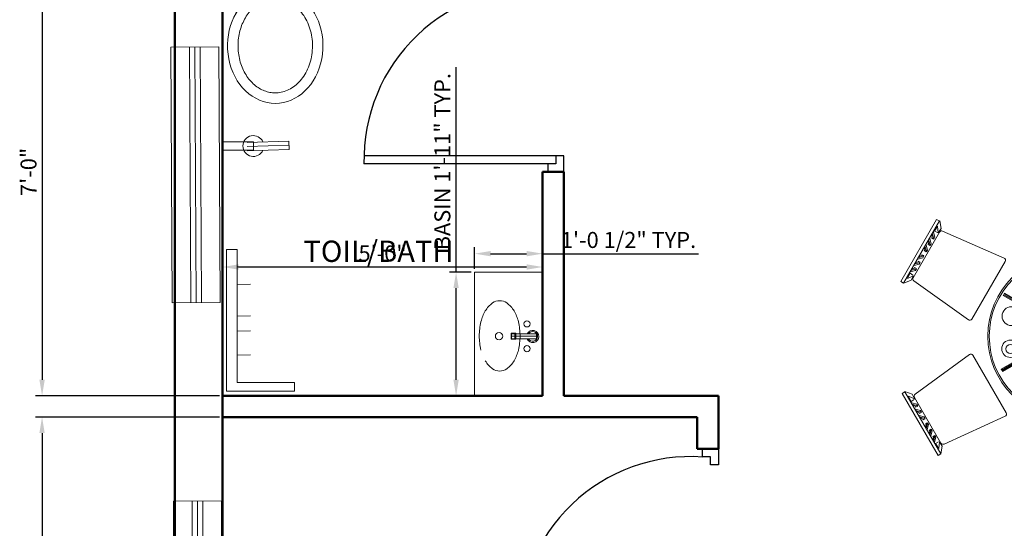
# Model space of a CAD drawing. Units: inches. Extents: x 108 to 1546, y -229 to 513.
# Tile 9 of 11: x 1167 to 1352, y 187 to 282. Entities that reach past the tile are written whole.
import ezdxf

# ---------------------------------------------------------------- set-up
doc = ezdxf.new("R2010")
doc.units = ezdxf.units.IN
for name, color, linetype, lineweight in [('A-ANNO-DIMS', 2, 'Continuous', 18), ('A-AREA-IDEN', 4, 'Continuous', 18), ('A-FLOR-FIXT', 9, 'Continuous', 18), ('A-FURN', 8, 'Continuous', 13), ('door', 1, 'Continuous', 25), ('wall', 7, 'Continuous', 50), ('WINDOW', 212, 'Continuous', 18)]:
    doc.layers.add(name, color=color, linetype=linetype, lineweight=lineweight)
doc.styles.get("Standard").update_dxf_attribs({"font": 'arial.ttf'})
doc.dimstyles.new('ISO-25', dxfattribs={"dimtxt": 3, "dimasz": 3, "dimexe": 1.25, "dimexo": 0.625, "dimtad": 1, "dimdec": 1, "dimlunit": 3, "dimtxsty": 'Standard', "dimcen": 2.5, "dimadec": 0, "dimazin": 0, "dimtfac": 1, "dimtdec": 1, "dimtmove": 0, "dimatfit": 3, "dimfxl": 1, "dimarcsym": 0})

# ---------------------------------------------------------------- blocks, each defined once
blk = doc.blocks.new('A$C45501D90')
for p, q in [((-242.2, 1133.5), (224, 1133.5)), ((-242.2, 1112.8), (-242.2, 1133.5)), ((224, 1112.8), (-242.2, 1112.8)), ((-242.2, 1111.2), (-202.3, 1079.2)), ((-203.9, 1106.4), (-165.6, 1108)), ((-168.8, 1080.8), (-203.9, 1106.4)), ((-165.6, 1108), (-167.2, 1085.6)), ((-156, 1109.6), (-132, 1085.6)), ((-119.3, 1085.6), (-143.2, 1108)), ((-143.2, 1108), (-133.6, 1108)), ((-133.6, 1108), (-122.5, 1098.4)), ((-122.5, 1098.4), (-119.3, 1101.6)), ((-119.3, 1101.6), (-117.7, 1087.2)), ((-108.1, 1109.6), (-84.1, 1085.6)), ((-71.4, 1085.6), (-95.3, 1108)), ((-95.3, 1108), (-85.7, 1108)), ((-85.7, 1108), (-74.6, 1098.4)), ((-74.6, 1098.4), (-71.4, 1101.6)), ((-71.4, 1101.6), (-69.8, 1087.2)), ((-60.2, 1109.6), (-36.2, 1085.6)), ((-23.5, 1085.6), (-47.4, 1108)), ((-47.4, 1108), (-37.8, 1108)), ((-37.8, 1108), (-26.7, 1098.4)), ((-26.7, 1098.4), (-23.5, 1101.6)), ((-23.5, 1101.6), (-21.9, 1087.2)), ((8.5, 1101.6), (6.9, 1087.2)), ((8.5, 1085.6), (32.4, 1108)), ((11.6, 1098.4), (8.5, 1101.6)), ((22.8, 1108), (11.6, 1098.4)), ((45.2, 1109.6), (21.2, 1085.6)), ((32.4, 1108), (22.8, 1108)), ((56.3, 1101.6), (54.8, 1087.2)), ((56.3, 1085.6), (80.3, 1108)), ((59.5, 1098.4), (56.3, 1101.6)), ((70.7, 1108), (59.5, 1098.4)), ((93.1, 1109.6), (69.1, 1085.6)), ((80.3, 1108), (70.7, 1108)), ((104.2, 1101.6), (102.6, 1087.2)), ((104.2, 1085.6), (128.2, 1108)), ((107.4, 1098.4), (104.2, 1101.6)), ((118.6, 1108), (107.4, 1098.4)), ((141, 1109.6), (117, 1085.6)), ((128.2, 1108), (118.6, 1108)), ((188.9, 1106.4), (150.5, 1108)), ((150.5, 1108), (152.1, 1085.6)), ((153.7, 1080.8), (188.9, 1106.4)), ((224, 1112.8), (187.3, 1079.2)), ((224, 1133.5), (224, 1112.8)), ((-197.3, 1061.6), (-238.9, 627.6)), ((-202.3, 1079.2), (-168.8, 1080.8)), ((161.8, 1076.1), (-181.4, 1076.1)), ((-132, 1085.6), (-119.3, 1085.6)), ((-84.1, 1085.6), (-71.4, 1085.6)), ((-36.2, 1085.6), (-23.5, 1085.6)), ((21.2, 1085.6), (8.5, 1085.6)), ((69.1, 1085.6), (56.3, 1085.6)), ((117, 1085.6), (104.2, 1085.6)), ((187.3, 1079.2), (153.7, 1080.8)), ((225.2, 627.8), (177.6, 1061.8)), ((842.6, 766.1), (860.5, 776.5)), ((860.5, 776.5), (1093.6, 372.8)), ((-1102.7, 357), (-869.7, 760.7)), ((-851.7, 750.4), (-1084.8, 346.6)), ((-863.7, 716.7), (-884.3, 684.4)), ((-869.7, 760.7), (-851.7, 750.4)), ((-859.2, 673.6), (-863.7, 716.7)), ((-848.7, 752.3), (-841, 701.8)), ((841.2, 765.3), (833.5, 714.8)), ((833.5, 714.8), (851.7, 686.6)), ((1075.7, 362.4), (842.6, 766.1)), ((851.7, 686.6), (856.2, 729.8)), ((856.2, 729.8), (876.7, 697.4)), ((-851, 678.1), (-1022.6, 380.9)), ((-897.5, 642.2), (-901.9, 641.1)), ((-901.9, 641.1), (-890.2, 632.5)), ((-895.4, 665), (-900.2, 656.7)), ((-900.2, 656.7), (-897.5, 642.2)), ((-888.1, 633.1), (-895.4, 665)), ((-890.4, 676.9), (-881.7, 644.2)), ((-881.7, 644.2), (-888.1, 633.1)), ((-884.3, 684.4), (-864.1, 674.6)), ((-841, 701.8), (-859.2, 673.6)), ((-431.1, 509), (-830.8, 684.8)), ((820.7, 701.7), (424.1, 520.7)), ((1012.8, 397.9), (841.2, 695.1)), ((876.7, 697.4), (856.6, 687.6)), ((882.9, 689.9), (874.2, 657.2)), ((874.2, 657.2), (880.6, 646.1)), ((880.6, 646.1), (887.9, 678)), ((894.4, 654.1), (882.7, 645.5)), ((887.9, 678), (892.7, 669.7)), ((892.7, 669.7), (890, 655.2)), ((890, 655.2), (894.4, 654.1)), ((906.9, 648.4), (898.1, 615.7)), ((-943.3, 582), (-948.1, 573.8)), ((-936, 550.1), (-943.3, 582)), ((-938.3, 593.9), (-929.6, 561.2)), ((-921.5, 600.8), (-925.8, 599.6)), ((-925.8, 599.6), (-914.2, 591)), ((-919.4, 623.5), (-924.2, 615.2)), ((-924.2, 615.2), (-921.5, 600.8)), ((-912, 591.6), (-919.4, 623.5)), ((-914.4, 635.4), (-905.6, 602.7)), ((-905.6, 602.7), (-912, 591.6)), ((-223, 610.1), (209.4, 610.1)), ((898.1, 615.7), (904.5, 604.6)), ((904.5, 604.6), (911.9, 636.5)), ((918.3, 612.6), (906.7, 604)), ((911.9, 636.5), (916.7, 628.2)), ((916.7, 628.2), (914, 613.8)), ((914, 613.8), (918.3, 612.6)), ((930.8, 606.9), (922.1, 574.2)), ((928.4, 563.1), (935.8, 595.1)), ((935.8, 595.1), (940.6, 586.8)), ((940.6, 586.8), (937.9, 572.3)), ((-951.9, 522.5), (-983.2, 512.9)), ((-983.2, 512.9), (-978.5, 521.2)), ((-978.5, 521.2), (-964.6, 526.1)), ((-964.6, 526.1), (-965.7, 530.5)), ((-965.7, 530.5), (-952.5, 524.7)), ((-958.3, 511.4), (-951.9, 522.5)), ((-945.4, 559.3), (-949.8, 558.1)), ((-949.8, 558.1), (-938.1, 549.6)), ((-948.1, 573.8), (-945.4, 559.3)), ((-929.6, 561.2), (-936, 550.1)), ((922.1, 574.2), (928.4, 563.1)), ((942.3, 571.1), (930.6, 562.6)), ((937.9, 572.3), (942.3, 571.1)), ((950.8, 524.4), (944.4, 535.5)), ((944.4, 535.5), (975.7, 525.9)), ((958.2, 543.5), (945, 537.7)), ((983.5, 515.7), (950.8, 524.4)), ((957.1, 539.1), (958.2, 543.5)), ((970.9, 534.2), (957.1, 539.1)), ((975.7, 525.9), (970.9, 534.2)), ((-1015, 461.2), (-982.3, 469.9)), ((-975.9, 481), (-1007.2, 471.4)), ((-1007.2, 471.4), (-1002.4, 479.7)), ((-1002.4, 479.7), (-988.5, 484.6)), ((-991, 502.7), (-958.3, 511.4)), ((-988.5, 484.6), (-989.7, 489)), ((-989.7, 489), (-976.5, 483.2)), ((-982.3, 469.9), (-975.9, 481)), ((-639.9, 111.9), (-423.7, 486.4)), ((-5.6, 508.7, 90.8), (0.4, 508.7, 90.8)), ((-5.6, 317.7, 90.8), (-5.6, 508.7, 90.8)), ((0.4, 508.7, 90.8), (0.4, 317.7, 90.8)), ((5.8, 317.7, 90.8), (5.8, 508.7, 90.8)), ((5.8, 508.7, 90.8), (11.8, 508.7, 90.8)), ((11.8, 508.7, 90.8), (11.8, 317.7, 90.8)), ((416.9, 498.2), (633.1, 123.7)), ((968.4, 494), (999.7, 484.4)), ((974.7, 483), (968.4, 494)), ((982.2, 502), (968.9, 496.2)), ((1007.4, 474.2), (974.7, 483)), ((981, 497.6), (982.2, 502)), ((994.9, 492.7), (981, 497.6)), ((998.7, 441.5), (992.3, 452.5)), ((992.3, 452.5), (1023.6, 443)), ((1006.1, 460.5), (992.9, 454.7)), ((999.7, 484.4), (994.9, 492.7)), ((1005, 456.2), (1006.1, 460.5)), ((1018.8, 451.3), (1005, 456.2)), ((1023.6, 443), (1018.8, 451.3)), ((-1060.1, 376.6), (-1042.3, 410.6)), ((-1020.4, 394.3), (-1060.1, 376.6)), ((-1042.3, 410.6), (-1023.8, 398.1)), ((-1038.9, 419.7), (-1006.2, 428.5)), ((-1035.8, 364.4), (-1020.4, 394.3)), ((-999.8, 439.5), (-1031.1, 430)), ((-1031.1, 430), (-1026.3, 438.3)), ((-1026.3, 438.3), (-1012.5, 443.1)), ((-1012.5, 443.1), (-1013.6, 447.5)), ((-1013.6, 447.5), (-1000.4, 441.7)), ((-1006.2, 428.5), (-999.8, 439.5)), ((1031.4, 432.7), (998.7, 441.5)), ((1028.3, 377.5), (1012.9, 407.3)), ((1012.9, 407.3), (1052.6, 389.6)), ((1034.8, 423.6), (1016.3, 411.1)), ((1052.6, 389.6), (1034.8, 423.6)), ((-1084.8, 346.6), (-1102.7, 357)), ((-1083.4, 345.8), (-1035.8, 364.4)), ((-1018, 360), (-663, 106.9)), ((-22.3, 329.1, 90.8), (-22.3, 344.6, 90.8)), ((-22.3, 344.6, 90.8), (-5.6, 344.6, 90.8)), ((-5.6, 329.1, 90.8), (-22.3, 329.1, 90.8)), ((0.4, 344.6, 90.8), (5.8, 344.6, 90.8)), ((5.8, 329.1, 90.8), (0.4, 329.1, 90.8)), ((11.8, 344.6, 90.8), (27.3, 344.6, 90.8)), ((27.3, 329.1, 90.8), (11.8, 329.1, 90.8)), ((27.3, 344.6, 90.8), (27.3, 329.1, 90.8)), ((656.3, 118.9), (1008.4, 377.1)), ((1075.9, 358.8), (1028.3, 377.5)), ((1093.6, 372.8), (1075.7, 362.4)), ((-436.3, 265.3, 90.8), (-433.3, 270.5, 90.8)), ((-270.9, 169.9, 90.8), (-436.3, 265.3, 90.8)), ((-433.3, 270.5, 90.8), (-267.9, 175, 90.8)), ((-430.6, 275.2, 90.8), (-427.6, 280.3, 90.8)), ((-265.2, 179.7, 90.8), (-430.6, 275.2, 90.8)), ((-427.6, 280.3, 90.8), (-262.3, 184.9, 90.8)), ((-175.3, 276.1, 90.8), (-104.8, 293.2, 90.8)), ((-103.3, 252.4, 90.8), (-175.3, 276.1, 90.8)), ((-104.8, 293.2, 90.8), (-85.5, 278.4, 90.8)), ((-85.5, 278.4, 90.8), (-52.1, 293.9, 90.8)), ((9.5, 276.1, 90.8), (-59.5, 246.5, 90.8)), ((-52.1, 293.9, 90.8), (9.5, 276.1, 90.8)), ((0.4, 317.7, 90.8), (-5.6, 317.7, 90.8)), ((11.8, 317.7, 90.8), (5.8, 317.7, 90.8)), ((134.3, 288, 90.8), (184.3, 235.5, 90.8)), ((149.7, 213.9, 90.8), (134.3, 288, 90.8)), ((255.2, 161.9, 90.8), (420.6, 257.3, 90.8)), ((420.6, 257.3, 90.8), (423.5, 252.2, 90.8)), ((-291.2, 188.5, 90.8), (-288.5, 193.1, 90.8)), ((-285.5, 198.3, 90.8), (-277.8, 211.7, 90.8)), ((-277.8, 211.7, 90.8), (-264.3, 204, 90.8)), ((-264.3, 204, 90.8), (-272.1, 190.5, 90.8)), ((-59.5, 246.5, 90.8), (-103.3, 252.4, 90.8)), ((166.5, 173, 90.8), (149.7, 213.9, 90.8)), ((184.3, 235.5, 90.8), (181.1, 211.4, 90.8)), ((181.1, 211.4, 90.8), (211.3, 190.3, 90.8)), ((423.5, 252.2, 90.8), (258.2, 156.7, 90.8)), ((260.9, 152, 90.8), (426.2, 247.5, 90.8)), ((429.2, 242.3, 90.8), (263.8, 146.9, 90.8)), ((426.2, 247.5, 90.8), (429.2, 242.3, 90.8)), ((-302.5, 168.8, 90.8), (-294.2, 183.3, 90.8)), ((-289.1, 161.1, 90.8), (-302.5, 168.8, 90.8)), ((-280.7, 175.5, 90.8), (-289.1, 161.1, 90.8)), ((-275.1, 185.4, 90.8), (-277.8, 180.7, 90.8)), ((-273.6, 117.6, 90.8), (-227.4, 162.1, 90.8)), ((-267.9, 175, 90.8), (-270.9, 169.9, 90.8)), ((-262.3, 184.9, 90.8), (-265.2, 179.7, 90.8)), ((-227.4, 162.1, 90.8), (-236.2, 87.5, 90.8)), ((226.7, 128.1, 90.8), (166.5, 173, 90.8)), ((211.3, 190.3, 90.8), (226.7, 128.1, 90.8)), ((258.2, 156.7, 90.8), (255.2, 161.9, 90.8)), ((256.6, 182, 90.8), (270.1, 189.8, 90.8)), ((265, 167.5, 90.8), (256.6, 182, 90.8)), ((263.8, 146.9, 90.8), (260.9, 152, 90.8)), ((270.7, 157.7, 90.8), (268, 162.4, 90.8)), ((270.1, 189.8, 90.8), (278.4, 175.3, 90.8)), ((281.4, 139.1, 90.8), (273.7, 152.5, 90.8)), ((281.4, 170.1, 90.8), (284.1, 165.5, 90.8)), ((294.9, 146.8, 90.8), (281.4, 139.1, 90.8)), ((287.1, 160.3, 90.8), (294.9, 146.8, 90.8)), ((-319.8, 2.1, 90.8), (-299.3, 71.7, 90.8)), ((-299.3, 71.7, 90.8), (-276.8, 80.9, 90.8)), ((-276.8, 80.9, 90.8), (-273.6, 117.6, 90.8)), ((-236.2, 87.5, 90.8), (-263.2, 52.5, 90.8)), ((-263.2, 52.5, 90.8), (-319.8, 2.1, 90.8)), ((242.9, -24.6, 90.8), (299.4, 25.9, 90.8)), ((299.4, 25.9, 90.8), (278.9, -43.7, 90.8)), ((207, -134.1, 90.8), (215.8, -59.5, 90.8)), ((215.8, -59.5, 90.8), (242.9, -24.6, 90.8)), ((256.4, -53, 90.8), (253.2, -89.7, 90.8)), ((278.9, -43.7, 90.8), (256.4, -53, 90.8)), ((-656.3, -118.9), (-1008.4, -377.1)), ((-416.9, -498.2), (-633.1, -123.7)), ((-449.6, -214.4, 90.8), (-284.2, -118.9, 90.8)), ((-281.2, -124.1, 90.8), (-446.6, -219.5, 90.8)), ((-315.2, -118.9, 90.8), (-301.8, -111.1, 90.8)), ((-307.5, -132.3, 90.8), (-315.2, -118.9, 90.8)), ((-301.8, -111.1, 90.8), (-294, -124.6, 90.8)), ((-284.2, -118.9, 90.8), (-281.2, -124.1, 90.8)), ((-247, -100.1, 90.8), (-186.8, -145, 90.8)), ((-231.7, -162.3, 90.8), (-247, -100.1, 90.8)), ((253.2, -89.7, 90.8), (207, -134.1, 90.8)), ((639.9, -111.9), (423.7, -486.4)), ((1018, -360), (663, -106.9)), ((-443.9, -224.2, 90.8), (-278.5, -128.7, 90.8)), ((-275.5, -133.9, 90.8), (-440.9, -229.4, 90.8)), ((-301.8, -142.1, 90.8), (-304.5, -137.5, 90.8)), ((-290.4, -161.8, 90.8), (-298.8, -147.3, 90.8)), ((-291, -129.7, 90.8), (-288.3, -134.4, 90.8)), ((-277, -154, 90.8), (-290.4, -161.8, 90.8)), ((-285.4, -139.5, 90.8), (-277, -154, 90.8)), ((-278.5, -128.7, 90.8), (-275.5, -133.9, 90.8)), ((-201.5, -183.4, 90.8), (-231.7, -162.3, 90.8)), ((-204.7, -207.6, 90.8), (-201.5, -183.4, 90.8)), ((-186.8, -145, 90.8), (-170.1, -185.9, 90.8)), ((-170.1, -185.9, 90.8), (-154.7, -260.1, 90.8)), ((241.9, -156.9, 90.8), (244.9, -151.7, 90.8)), ((407.3, -252.4, 90.8), (241.9, -156.9, 90.8)), ((244, -176, 90.8), (251.7, -162.5, 90.8)), ((257.4, -183.7, 90.8), (244, -176, 90.8)), ((244.9, -151.7, 90.8), (410.3, -247.2, 90.8)), ((247.6, -147.1, 90.8), (250.6, -141.9, 90.8)), ((413, -242.5, 90.8), (247.6, -147.1, 90.8)), ((250.6, -141.9, 90.8), (415.9, -237.4, 90.8)), ((254.7, -157.4, 90.8), (257.4, -152.7, 90.8)), ((265.2, -170.3, 90.8), (257.4, -183.7, 90.8)), ((260.4, -147.6, 90.8), (268.7, -133.1, 90.8)), ((270.8, -160.5, 90.8), (268.1, -165.1, 90.8)), ((268.7, -133.1, 90.8), (282.2, -140.8, 90.8)), ((282.2, -140.8, 90.8), (273.8, -155.3, 90.8)), ((-446.6, -219.5, 90.8), (-449.6, -214.4, 90.8)), ((-440.9, -229.4, 90.8), (-443.9, -224.2, 90.8)), ((-154.7, -260.1, 90.8), (-204.7, -207.6, 90.8)), ((-29.8, -248.2, 90.8), (39.2, -218.5, 90.8)), ((31.8, -266, 90.8), (-29.8, -248.2, 90.8)), ((65.2, -250.4, 90.8), (31.8, -266, 90.8)), ((39.2, -218.5, 90.8), (83, -224.4, 90.8)), ((84.4, -265.2, 90.8), (65.2, -250.4, 90.8)), ((83, -224.4, 90.8), (154.9, -248.2, 90.8)), ((154.9, -248.2, 90.8), (84.4, -265.2, 90.8)), ((410.3, -247.2, 90.8), (407.3, -252.4, 90.8)), ((415.9, -237.4, 90.8), (413, -242.5, 90.8)), ((-47.6, -316.6, 90.8), (-47.6, -301.1, 90.8)), ((-47.6, -301.1, 90.8), (-32.1, -301.1, 90.8)), ((-32.1, -316.6, 90.8), (-47.6, -316.6, 90.8)), ((-32.1, -480.7, 90.8), (-32.1, -289.8, 90.8)), ((-32.1, -289.8, 90.8), (-26.1, -289.8, 90.8)), ((-26.1, -289.8, 90.8), (-26.1, -480.7, 90.8)), ((-26.1, -301.1, 90.8), (-20.8, -301.1, 90.8)), ((-20.8, -316.6, 90.8), (-26.1, -316.6, 90.8)), ((-20.8, -480.7, 90.8), (-20.8, -289.8, 90.8)), ((-20.8, -289.8, 90.8), (-14.8, -289.8, 90.8)), ((-14.8, -289.8, 90.8), (-14.8, -480.7, 90.8)), ((-14.8, -301.1, 90.8), (1.9, -301.1, 90.8)), ((1.9, -316.6, 90.8), (-14.8, -316.6, 90.8)), ((1.9, -301.1, 90.8), (1.9, -316.6, 90.8)), ((-1093.6, -372.8), (-1075.7, -362.4)), ((-860.5, -776.5), (-1093.6, -372.8)), ((-1075.9, -358.8), (-1028.3, -377.5)), ((-1075.7, -362.4), (-842.6, -766.1)), ((-1028.3, -377.5), (-1012.9, -407.3)), ((851, -678.1), (1022.6, -380.9)), ((851.7, -750.4), (1084.8, -346.6)), ((1102.7, -357), (869.7, -760.7)), ((1035.8, -364.4), (1020.4, -394.3)), ((1020.4, -394.3), (1060.1, -376.6)), ((1083.4, -345.8), (1035.8, -364.4)), ((1060.1, -376.6), (1042.3, -410.6)), ((1084.8, -346.6), (1102.7, -357)), ((-1052.6, -389.6), (-1034.8, -423.6)), ((-1012.9, -407.3), (-1052.6, -389.6)), ((-1034.8, -423.6), (-1016.3, -411.1)), ((-1031.4, -432.7), (-998.7, -441.5)), ((-1023.6, -443), (-1018.8, -451.3)), ((-992.3, -452.5), (-1023.6, -443)), ((-1012.8, -397.9), (-841.2, -695.1)), ((-998.7, -441.5), (-992.3, -452.5)), ((1006.2, -428.5), (999.8, -439.5)), ((999.8, -439.5), (1031.1, -430)), ((1013.6, -447.5), (1000.4, -441.7)), ((1038.9, -419.7), (1006.2, -428.5)), ((1026.3, -438.3), (1012.5, -443.1)), ((1012.5, -443.1), (1013.6, -447.5)), ((1042.3, -410.6), (1023.8, -398.1)), ((1031.1, -430), (1026.3, -438.3)), ((-1018.8, -451.3), (-1005, -456.2)), ((-1007.4, -474.2), (-974.7, -483)), ((-1006.1, -460.5), (-992.9, -454.7)), ((-1005, -456.2), (-1006.1, -460.5)), ((-968.4, -494), (-999.7, -484.4)), ((-999.7, -484.4), (-994.9, -492.7)), ((-994.9, -492.7), (-981, -497.6)), ((-982.2, -502), (-968.9, -496.2)), ((-981, -497.6), (-982.2, -502)), ((-974.7, -483), (-968.4, -494)), ((-26.1, -480.7, 90.8), (-32.1, -480.7, 90.8)), ((-14.8, -480.7, 90.8), (-20.8, -480.7, 90.8)), ((431.1, -509), (830.8, -684.8)), ((958.3, -511.4), (951.9, -522.5)), ((991, -502.7), (958.3, -511.4)), ((982.3, -469.9), (975.9, -481)), ((975.9, -481), (1007.2, -471.4)), ((989.7, -489), (976.5, -483.2)), ((1015, -461.2), (982.3, -469.9)), ((1002.4, -479.7), (988.5, -484.6)), ((988.5, -484.6), (989.7, -489)), ((1007.2, -471.4), (1002.4, -479.7)), ((-983.5, -515.7), (-950.8, -524.4)), ((-944.4, -535.5), (-975.7, -525.9)), ((-975.7, -525.9), (-970.9, -534.2)), ((-970.9, -534.2), (-957.1, -539.1)), ((-958.2, -543.5), (-945, -537.7)), ((-957.1, -539.1), (-958.2, -543.5)), ((-950.8, -524.4), (-944.4, -535.5)), ((-942.3, -571.1), (-930.6, -562.6)), ((-937.9, -572.3), (-942.3, -571.1)), ((-940.6, -586.8), (-937.9, -572.3)), ((-928.4, -563.1), (-935.8, -595.1)), ((-930.8, -606.9), (-922.1, -574.2)), ((-922.1, -574.2), (-928.4, -563.1)), ((-820.7, -701.7), (-424.1, -520.7)), ((929.6, -561.2), (936, -550.1)), ((938.3, -593.9), (929.6, -561.2)), ((936, -550.1), (943.3, -582)), ((949.8, -558.1), (938.1, -549.6)), ((943.3, -582), (948.1, -573.8)), ((945.4, -559.3), (949.8, -558.1)), ((948.1, -573.8), (945.4, -559.3)), ((951.9, -522.5), (983.2, -512.9)), ((965.7, -530.5), (952.5, -524.7)), ((978.5, -521.2), (964.6, -526.1)), ((964.6, -526.1), (965.7, -530.5)), ((983.2, -512.9), (978.5, -521.2)), ((-935.8, -595.1), (-940.6, -586.8)), ((-918.3, -612.6), (-906.7, -604)), ((-914, -613.8), (-918.3, -612.6)), ((-916.7, -628.2), (-914, -613.8)), ((-911.9, -636.5), (-916.7, -628.2)), ((-904.5, -604.6), (-911.9, -636.5)), ((-906.9, -648.4), (-898.1, -615.7)), ((-898.1, -615.7), (-904.5, -604.6)), ((-229.3, -629.3), (-181.8, -1063.3)), ((-225.2, -627.8), (-177.6, -1061.8)), ((218.9, -611.6), (-213.5, -611.6)), ((223, -610.1), (-209.4, -610.1)), ((193.2, -1063.1), (234.8, -629.1)), ((197.3, -1061.6), (238.9, -627.6)), ((881.7, -644.2), (888.1, -633.1)), ((888.1, -633.1), (895.4, -665)), ((901.9, -641.1), (890.2, -632.5)), ((905.6, -602.7), (912, -591.6)), ((914.4, -635.4), (905.6, -602.7)), ((912, -591.6), (919.4, -623.5)), ((925.8, -599.6), (914.2, -591)), ((919.4, -623.5), (924.2, -615.2)), ((921.5, -600.8), (925.8, -599.6)), ((924.2, -615.2), (921.5, -600.8)), ((-894.4, -654.1), (-882.7, -645.5)), ((-890, -655.2), (-894.4, -654.1)), ((-892.7, -669.7), (-890, -655.2)), ((-887.9, -678), (-892.7, -669.7)), ((-880.6, -646.1), (-887.9, -678)), ((-882.9, -689.9), (-874.2, -657.2)), ((-874.2, -657.2), (-880.6, -646.1)), ((-876.7, -697.4), (-856.6, -687.6)), ((-856.2, -729.8), (-876.7, -697.4)), ((-851.7, -686.6), (-856.2, -729.8)), ((-833.5, -714.8), (-851.7, -686.6)), ((841, -701.8), (859.2, -673.6)), ((848.7, -752.3), (841, -701.8)), ((859.2, -673.6), (863.7, -716.7)), ((863.7, -716.7), (884.3, -684.4)), ((884.3, -684.4), (864.1, -674.6)), ((890.4, -676.9), (881.7, -644.2)), ((895.4, -665), (900.2, -656.7)), ((897.5, -642.2), (901.9, -641.1)), ((900.2, -656.7), (897.5, -642.2)), ((-842.6, -766.1), (-860.5, -776.5)), ((-841.2, -765.3), (-833.5, -714.8)), ((869.7, -760.7), (851.7, -750.4)), ((-231.3, -1112.7), (-191.4, -1080.8)), ((-227.2, -1111.2), (-187.3, -1079.2)), ((-157.9, -1082.4), (-193, -1107.9)), ((-191.4, -1080.8), (-157.9, -1082.4)), ((-153.7, -1080.8), (-188.9, -1106.4)), ((-187.3, -1079.2), (-153.7, -1080.8)), ((-165.9, -1077.6), (177.3, -1077.6)), ((-161.8, -1076.1), (181.4, -1076.1)), ((-154.7, -1109.5), (-156.3, -1087.1)), ((-150.5, -1108), (-152.1, -1085.6)), ((-145.1, -1111.1), (-121.1, -1087.1)), ((-141, -1109.6), (-117, -1085.6)), ((-108.4, -1087.1), (-132.3, -1109.5)), ((-104.2, -1085.6), (-128.2, -1108)), ((-121.1, -1087.1), (-108.4, -1087.1)), ((-117, -1085.6), (-104.2, -1085.6)), ((-108.4, -1103.1), (-106.8, -1088.7)), ((-104.2, -1101.6), (-102.6, -1087.2)), ((-97.2, -1111.1), (-73.2, -1087.1)), ((-93.1, -1109.6), (-69.1, -1085.6)), ((-60.5, -1087.1), (-84.4, -1109.5)), ((-56.3, -1085.6), (-80.3, -1108)), ((-73.2, -1087.1), (-60.5, -1087.1)), ((-69.1, -1085.6), (-56.3, -1085.6)), ((-60.5, -1103.1), (-58.9, -1088.7)), ((-56.3, -1101.6), (-54.8, -1087.2)), ((-49.3, -1111.1), (-25.3, -1087.1)), ((-45.2, -1109.6), (-21.2, -1085.6)), ((-12.6, -1087.1), (-36.5, -1109.5)), ((-8.5, -1085.6), (-32.4, -1108)), ((-25.3, -1087.1), (-12.6, -1087.1)), ((-21.2, -1085.6), (-8.5, -1085.6)), ((-12.6, -1103.1), (-11, -1088.7)), ((-8.5, -1101.6), (-6.9, -1087.2)), ((19.4, -1103.1), (17.8, -1088.7)), ((19.4, -1087.1), (43.3, -1109.5)), ((32.1, -1087.1), (19.4, -1087.1)), ((23.5, -1101.6), (21.9, -1087.2)), ((23.5, -1085.6), (47.4, -1108)), ((36.2, -1085.6), (23.5, -1085.6)), ((56.1, -1111.1), (32.1, -1087.1)), ((60.2, -1109.6), (36.2, -1085.6)), ((67.3, -1103.1), (65.7, -1088.7)), ((67.3, -1087.1), (91.2, -1109.5)), ((80, -1087.1), (67.3, -1087.1)), ((71.4, -1101.6), (69.8, -1087.2)), ((71.4, -1085.6), (95.3, -1108)), ((84.1, -1085.6), (71.4, -1085.6)), ((104, -1111.1), (80, -1087.1)), ((108.1, -1109.6), (84.1, -1085.6)), ((115.1, -1103.1), (113.6, -1088.7)), ((115.1, -1087.1), (139.1, -1109.5)), ((127.9, -1087.1), (115.1, -1087.1)), ((119.3, -1101.6), (117.7, -1087.2)), ((119.3, -1085.6), (143.2, -1108)), ((132, -1085.6), (119.3, -1085.6)), ((151.9, -1111.1), (127.9, -1087.1)), ((156, -1109.6), (132, -1085.6)), ((161.4, -1109.5), (163, -1087.1)), ((198.2, -1080.8), (164.6, -1082.4)), ((164.6, -1082.4), (199.8, -1107.9)), ((165.6, -1108), (167.2, -1085.6)), ((202.3, -1079.2), (168.8, -1080.8)), ((168.8, -1080.8), (203.9, -1106.4)), ((238.1, -1112.7), (198.2, -1080.8)), ((242.2, -1111.2), (202.3, -1079.2)), ((-228.1, -1114.3), (238.1, -1114.3)), ((-228.1, -1135), (-228.1, -1114.3)), ((238.1, -1135), (-228.1, -1135)), ((-224, -1112.8), (242.2, -1112.8)), ((-224, -1133.5), (-224, -1112.8)), ((242.2, -1133.5), (-224, -1133.5)), ((-193, -1107.9), (-154.7, -1109.5)), ((-188.9, -1106.4), (-150.5, -1108)), ((-132.3, -1109.5), (-122.7, -1109.5)), ((-128.2, -1108), (-118.6, -1108)), ((-122.7, -1109.5), (-111.6, -1099.9)), ((-118.6, -1108), (-107.4, -1098.4)), ((-111.6, -1099.9), (-108.4, -1103.1)), ((-107.4, -1098.4), (-104.2, -1101.6)), ((-84.4, -1109.5), (-74.8, -1109.5)), ((-80.3, -1108), (-70.7, -1108)), ((-74.8, -1109.5), (-63.7, -1099.9)), ((-70.7, -1108), (-59.5, -1098.4)), ((-63.7, -1099.9), (-60.5, -1103.1)), ((-59.5, -1098.4), (-56.3, -1101.6)), ((-36.5, -1109.5), (-26.9, -1109.5)), ((-32.4, -1108), (-22.8, -1108)), ((-26.9, -1109.5), (-15.8, -1099.9)), ((-22.8, -1108), (-11.6, -1098.4)), ((-15.8, -1099.9), (-12.6, -1103.1)), ((-11.6, -1098.4), (-8.5, -1101.6)), ((22.6, -1099.9), (19.4, -1103.1)), ((33.7, -1109.5), (22.6, -1099.9)), ((26.7, -1098.4), (23.5, -1101.6)), ((37.8, -1108), (26.7, -1098.4)), ((43.3, -1109.5), (33.7, -1109.5)), ((47.4, -1108), (37.8, -1108)), ((70.4, -1099.9), (67.3, -1103.1)), ((81.6, -1109.5), (70.4, -1099.9)), ((74.6, -1098.4), (71.4, -1101.6)), ((85.7, -1108), (74.6, -1098.4)), ((91.2, -1109.5), (81.6, -1109.5)), ((95.3, -1108), (85.7, -1108)), ((118.3, -1099.9), (115.1, -1103.1)), ((129.5, -1109.5), (118.3, -1099.9)), ((122.5, -1098.4), (119.3, -1101.6)), ((133.6, -1108), (122.5, -1098.4)), ((139.1, -1109.5), (129.5, -1109.5)), ((143.2, -1108), (133.6, -1108)), ((199.8, -1107.9), (161.4, -1109.5)), ((203.9, -1106.4), (165.6, -1108)), ((238.1, -1114.3), (238.1, -1135)), ((242.2, -1112.8), (242.2, -1133.5))]:
    blk.add_line(p, q)
for centre, radius in [((0, 0), 537), ((0, 0), 527), ((-94.8, 394.7, 90.8), 61.3), ((96.9, 390, 90.8), 56.9), ((95.5, 390.7, 90.8), 29.4), ((-282.3, 294.7, 90.8), 56.9), ((-283.5, 293.9, 90.8), 29.4), ((277.2, 277.6, 90.8), 61.3), ((-382.1, 131.1, 90.8), 61.3), ((369, 109.3, 90.8), 56.9), ((368.9, 110.8, 90.8), 29.4), ((-389.3, -81.3, 90.8), 56.9), ((-389.2, -82.8, 90.8), 29.4), ((361.8, -103.1, 90.8), 61.3), ((-297.5, -249.6, 90.8), 61.3), ((261.9, -266.7, 90.8), 56.9), ((263.2, -265.9, 90.8), 29.4), ((-117.2, -362, 90.8), 56.9), ((74.4, -366.7, 90.8), 61.3), ((-115.9, -362.7, 90.8), 29.4)]:
    blk.add_circle(centre, radius)
for centre, radius, start, end in [((-181.4, 1060.1), 16, 90, 174.51988), ((161.8, 1060.1), 16, 6.25717, 90), ((-837.2, 670.1), 16, 66.25717, 150), ((827.4, 687.1), 16, 30, 114.51988), ((-223, 626.1), 16, 174.51988, 270), ((209.4, 626.1), 16, 270, 6.25717), ((430.7, 506.2), 16, 114.51988, 210), ((-437.5, 494.4), 16, 330, 66.25717), ((999, 389.9), 16, 306.25717, 30), ((-1008.8, 373), 16, 150, 234.51988), ((-77.3, 270.2, 90.8), 44.6, 195.93383, 342.9389), ((-77.3, 270.2, 90.8), 44.6, 25.85584, 153.33587), ((178.1, 200.3, 90.8), 44.6, 135.93383, 282.9389), ((178.1, 200.3, 90.8), 44.6, 325.85584, 93.33587), ((-265.7, 83.9, 90.8), 44.6, 85.85584, 213.33587), ((-653.7, 119.9), 16, 234.51988, 330), ((-265.7, 83.9, 90.8), 44.6, 255.93383, 42.9389), ((646.9, 131.7), 16, 210, 306.25717), ((245.3, -55.9, 90.8), 44.6, 75.93383, 222.9389), ((245.3, -55.9, 90.8), 44.6, 265.85584, 33.33587), ((-646.9, -131.7), 16, 30, 126.25717), ((-198.5, -172.3, 90.8), 44.6, 315.93383, 102.9389), ((653.7, -119.9), 16, 54.51988, 150), ((-198.5, -172.3, 90.8), 44.6, 145.85584, 273.33587), ((57, -242.2, 90.8), 44.6, 15.93383, 162.9389), ((57, -242.2, 90.8), 44.6, 205.85584, 333.33587), ((-999, -389.9), 16, 126.25717, 210), ((1008.8, -373), 16, 330, 54.51988), ((-430.7, -506.2), 16, 294.51988, 30), ((437.5, -494.4), 16, 150, 246.25717), ((-213.5, -627.6), 16, 90, 186.25717), ((-209.4, -626.1), 16, 90, 186.25717), ((218.9, -627.6), 16, 354.51988, 90), ((223, -626.1), 16, 354.51988, 90), ((-827.4, -687.1), 16, 210, 294.51988), ((837.2, -670.1), 16, 246.25717, 330), ((-165.9, -1061.6), 16, 186.25717, 270), ((-161.8, -1060.1), 16, 186.25717, 270), ((177.3, -1061.6), 16, 270, 354.51988), ((181.4, -1060.1), 16, 270, 354.51988)]:
    blk.add_arc(centre, radius, start, end)
blk = doc.blocks.new('A$C7C8779AE')
for p, q in [((0, 0.7405), (0, 0.5605)), ((0.5, 0.7405), (0, 0.7405)), ((0.47, 0.7105), (0.03, 0.7105)), ((0.03, 0.7105), (0.03, 0.5905)), ((0.47, 0.5905), (0.47, 0.7105)), ((0.5, 0.5605), (0.5, 0.7405)), ((0.093, 0.6405), (0.063, 0.5905)), ((0.11, 0.6105), (0.08, 0.5605)), ((0.093, 0.6405), (0.407, 0.6405)), ((0.11, 0.6105), (0.39, 0.6105)), ((0.42, 0.5605), (0.39, 0.6105)), ((0.437, 0.5905), (0.407, 0.6405)), ((0.03, 0.5905), (0.063, 0.5905)), ((0.437, 0.5905), (0.47, 0.5905)), ((0, 0.5605), (0.08, 0.5605)), ((0.1497, 0.557), (0.1497, 0.5203)), ((0.1497, 0.557), (0.3514, 0.557)), ((0.3514, 0.557), (0.3514, 0.5203)), ((0.42, 0.5605), (0.5, 0.5605)), ((0.1997, 0.507), (0.1997, 0.4879)), ((0.1997, 0.507), (0.3014, 0.507)), ((0.3014, 0.507), (0.3014, 0.4879))]:
    blk.add_line(p, q)
for centre, start, end in [((-0.0386, 0.4613), 344.642, 68.7339), ((0.5386, 0.4613), 111.2661, 195.358)]:
    blk.add_arc(centre, 0.1064, start, end)
blk.add_ellipse((0.2506, 0.2744), major_axis=(0, 0.2744), ratio=0.828948, start_param=0.459479, end_param=5.823706)
blk.add_open_spline([(0.1997, 0.4879), (0.1697, 0.474), (0.1642, 0.4702), (0.1512, 0.4602), (0.1438, 0.4535), (0.1298, 0.4388), (0.1233, 0.4306), (0.1111, 0.4131), (0.1055, 0.4037), (0.0956, 0.3838), (0.0912, 0.3733), (0.0838, 0.3516), (0.0808, 0.3403), (0.0762, 0.3172), (0.0746, 0.3055), (0.073, 0.2817), (0.0729, 0.2698), (0.0743, 0.246), (0.0758, 0.2342), (0.0801, 0.2111), (0.0831, 0.1998), (0.0903, 0.1779), (0.0945, 0.1673), (0.1043, 0.1473), (0.1098, 0.1378), (0.1218, 0.12), (0.1283, 0.1118), (0.1421, 0.0968), (0.1494, 0.09), (0.1646, 0.078), (0.1725, 0.0728), (0.1887, 0.064), (0.1969, 0.0603), (0.2137, 0.0547), (0.2222, 0.0527), (0.2392, 0.0502), (0.2478, 0.0498), (0.2664, 0.0505), (0.2764, 0.052), (0.2963, 0.0573), (0.3061, 0.061), (0.3253, 0.0707), (0.3346, 0.0766), (0.3525, 0.0906), (0.3611, 0.0987), (0.3771, 0.1169), (0.3845, 0.127), (0.3978, 0.1488), (0.4037, 0.1605), (0.4137, 0.1853), (0.4178, 0.1983), (0.424, 0.2251), (0.4261, 0.2389), (0.4282, 0.2668), (0.4283, 0.2809), (0.4262, 0.3088), (0.4241, 0.3226), (0.418, 0.3495), (0.414, 0.3625), (0.404, 0.3873), (0.3982, 0.3991), (0.385, 0.421), (0.3776, 0.4311), (0.3617, 0.4494), (0.3531, 0.4575), (0.3382, 0.4693), (0.3321, 0.4736), (0.3014, 0.4879)], degree=3, knots=[0.459479, 0.459479, 0.459479, 0.459479, 0.567422, 0.567422, 0.720865, 0.720865, 0.874307, 0.874307, 1.02775, 1.02775, 1.181192, 1.181192, 1.334635, 1.334635, 1.488077, 1.488077, 1.64152, 1.64152, 1.794963, 1.794963, 1.948405, 1.948405, 2.101848, 2.101848, 2.25529, 2.25529, 2.408733, 2.408733, 2.562175, 2.562175, 2.715618, 2.715618, 2.86906, 2.86906, 3.022503, 3.022503, 3.175946, 3.175946, 3.356457, 3.356457, 3.536968, 3.536968, 3.717479, 3.717479, 3.89799, 3.89799, 4.078501, 4.078501, 4.259012, 4.259012, 4.439523, 4.439523, 4.620035, 4.620035, 4.800546, 4.800546, 4.981057, 4.981057, 5.161568, 5.161568, 5.342079, 5.342079, 5.52259, 5.52259, 5.703101, 5.703101, 5.823706, 5.823706, 5.823706, 5.823706])
blk = doc.blocks.new('WINDOW-48X9')
for p, q in [((0, 9), (0, 0)), ((0, 9), (48, 9)), ((48, 9), (48, 0)), ((0, 5.5), (48, 5.5)), ((0, 4.5), (48, 4.5)), ((0, 3.5), (48, 3.5)), ((0, 0), (48, 0))]:
    blk.add_line(p, q)
blk = doc.blocks.new('DOOR-SWING-36')
for p, q in [((1.5, 1.5), (1.5, 37.5)), ((3, 1.5), (3, 37.5)), ((0, 3), (0, 0)), ((1.5, 3), (0, 3)), ((1.5, 1.5), (1.5, 3)), ((34.5, 1.5), (34.5, 3)), ((34.5, 3), (36, 3)), ((36, 3), (36, 0)), ((3, 1.5), (1.5, 1.5)), ((3, 0), (3, 1.5)), ((33, 0), (33, 1.5)), ((33, 1.5), (34.5, 1.5)), ((0, 0), (3, 0)), ((36, 0), (33, 0))]:
    blk.add_line(p, q)
blk.add_arc((2.25, 5.18), 32.32, 356.1244, 91.3295)
blk = doc.blocks.new('LAVATORY-COMPACT')
for p, q in [((12.75, 23.17), (0, 23.17)), ((0, 23.17), (0, 0)), ((0, 23.17), (0, 0)), ((12.75, 23.17), (12.75, 0)), ((7.76, 11.74), (6.84, 11.74)), ((6.84, 11.74), (6.84, 10.58)), ((11.59, 11.62), (6.95, 11.62)), ((6.95, 11.62), (6.95, 10.7)), ((11.59, 11.16), (6.95, 11.16)), ((7.53, 11.62), (7.53, 10.7)), ((7.76, 11.74), (7.76, 10.58)), ((11.59, 11.62), (11.59, 10.7)), ((7.76, 10.58), (6.84, 10.58)), ((11.59, 10.7), (6.95, 10.7)), ((12.75, 0), (0, 0))]:
    blk.add_line(p, q)
for centre, radius in [((9.83, 13.48), 0.579), ((4.59, 11.16), 0.69), ((9.83, 8.84), 0.579)]:
    blk.add_circle(centre, radius)
for centre, radius, start, end in [((6.18, 13.48), 4.82, 125.5822, 149.9314), ((4.71, 15.53), 2.3, 90, 125.5822), ((4.71, 15.53), 2.3, 54.4178, 90), ((3.24, 13.48), 4.82, 30.0686, 54.4178), ((8.53, 12.12), 7.54, 149.9314, 166.5147), ((0.89, 12.12), 7.54, 13.4853, 30.0686), ((12.25, 11.22), 11.37, 166.5147, 180), ((-2.84, 11.22), 11.37, 360, 13.4853), ((12.25, 11.22), 11.37, 180, 193.4853), ((-2.84, 11.22), 11.37, 346.5147, 0), ((10.9, 11.12), 1.15, 201.7425, 154.2331), ((10.9, 11.12), 0.92, 207.632, 147.0256), ((0.89, 10.33), 7.54, 329.9314, 346.5147), ((6.18, 8.97), 4.82, 210.0686, 234.4178), ((3.24, 8.97), 4.82, 305.5822, 329.9314), ((4.71, 6.91), 2.3, 234.4178, 270), ((4.71, 6.91), 2.3, 270, 305.5822)]:
    blk.add_arc(centre, radius, start, end)
blk = doc.blocks.new('BATH-CORNER-RACK')
for p, q in [((2.03, 23.32), (4.51, 23.38)), ((2.03, 20.06), (4.51, 20.12)), ((2.03, 14.08), (4.51, 14.14)), ((2.03, 11.27), (4.51, 11.33)), ((2.03, 6.76), (4.51, 6.83))]:
    blk.add_line(p, q)
for points in [[(2.03, 1.66), (2.03, 26.63), (0, 26.63), (0, 0), (2.03, 0)], [(0, 1.66), (0, 1.66), (0, 0), (12.78, 0), (12.78, 1.66), (2.03, 1.66)]]:
    blk.add_lwpolyline(points)
blk = doc.blocks.new('*D60')
at = {"layer": 'A-ANNO-DIMS', "color": 0, "lineweight": -2, "transparency": 16777216}
for p, q in [((1248.72, 234.65), (1248.72, 273.12)), ((1251.57, 234.65), (1247.47, 234.65)), ((1248.72, 214.47), (1248.72, 231.65)), ((1251.57, 211.47), (1247.47, 211.47))]:
    blk.add_line(p, q, dxfattribs=at)
at = {"layer": 'A-ANNO-DIMS', "color": 0, "transparency": 16777216}
for points in [[(1248.22, 231.65), (1249.22, 231.65), (1248.72, 234.65)], [(1248.22, 214.47), (1249.22, 214.47), (1248.72, 211.47)]]:
    blk.add_solid(points, dxfattribs=at)
at = {"layer": 'Defpoints', "color": 0, "transparency": 16777216}
for p in [(1248.72, 234.65), (1252.19, 234.65), (1252.19, 211.47)]:
    blk.add_point(p, dxfattribs=at)
at = {"layer": 'A-ANNO-DIMS', "color": 0, "transparency": 16777216, "insert": (1246.54, 255.38), "char_height": 3, "attachment_point": 5, "rotation": 90}
blk.add_mtext('BASIN 1\'-11" TYP.', dxfattribs=at)
blk = doc.blocks.new('*D61')
at = {"layer": 'A-ANNO-DIMS', "color": 0, "lineweight": -2, "transparency": 16777216}
for p, q in [((1252.19, 235.27), (1252.19, 239.37)), ((1264.94, 235.27), (1264.94, 239.37)), ((1255.19, 238.12), (1261.94, 238.12)), ((1264.94, 238.12), (1294.18, 238.12))]:
    blk.add_line(p, q, dxfattribs=at)
at = {"layer": 'A-ANNO-DIMS', "color": 0, "transparency": 16777216}
for points in [[(1255.19, 238.62), (1255.19, 237.62), (1252.19, 238.12)], [(1261.94, 238.62), (1261.94, 237.62), (1264.94, 238.12)]]:
    blk.add_solid(points, dxfattribs=at)
at = {"layer": 'Defpoints', "color": 0, "transparency": 16777216}
for p in [(1264.94, 238.12), (1252.19, 234.65), (1264.94, 234.65)]:
    blk.add_point(p, dxfattribs=at)
at = {"layer": 'A-ANNO-DIMS', "color": 0, "transparency": 16777216, "insert": (1281.06, 240.3), "char_height": 3, "attachment_point": 5}
blk.add_mtext('1\'-0 1/2" TYP.', dxfattribs=at)
blk = doc.blocks.new('*D103')
at = {"layer": 'A-ANNO-DIMS', "color": 0, "lineweight": -2, "transparency": 16777216}
for p, q in [((1204.94, 212.09), (1204.94, 236.87)), ((1264.94, 212.09), (1264.94, 236.87)), ((1207.94, 235.62), (1261.94, 235.62))]:
    blk.add_line(p, q, dxfattribs=at)
at = {"layer": 'A-ANNO-DIMS', "color": 0, "transparency": 16777216}
for points in [[(1207.94, 236.12), (1207.94, 235.12), (1204.94, 235.62)], [(1261.94, 236.12), (1261.94, 235.12), (1264.94, 235.62)]]:
    blk.add_solid(points, dxfattribs=at)
at = {"layer": 'Defpoints', "color": 0, "transparency": 16777216}
for p in [(1264.94, 235.62), (1204.94, 211.47), (1264.94, 211.47)]:
    blk.add_point(p, dxfattribs=at)
at = {"layer": 'A-ANNO-DIMS', "color": 0, "transparency": 16777216, "insert": (1234.94, 237.78), "char_height": 3, "attachment_point": 5}
blk.add_mtext('5\'-0"', dxfattribs=at)
blk = doc.blocks.new('*D106')
at = {"layer": 'A-ANNO-DIMS', "color": 0, "lineweight": -2, "transparency": 16777216}
for p, q in [((1204.32, 295.47), (1169.82, 295.47)), ((1171.07, 292.47), (1171.07, 214.47)), ((1204.32, 211.47), (1169.82, 211.47))]:
    blk.add_line(p, q, dxfattribs=at)
at = {"layer": 'A-ANNO-DIMS', "color": 0, "transparency": 16777216}
for points in [[(1170.57, 292.47), (1171.57, 292.47), (1171.07, 295.47)], [(1170.57, 214.47), (1171.57, 214.47), (1171.07, 211.47)]]:
    blk.add_solid(points, dxfattribs=at)
at = {"layer": 'Defpoints', "color": 0, "transparency": 16777216}
for p in [(1204.94, 295.47), (1171.07, 211.47), (1204.94, 211.47)]:
    blk.add_point(p, dxfattribs=at)
at = {"layer": 'A-ANNO-DIMS', "color": 0, "transparency": 16777216, "insert": (1168.92, 253.47), "char_height": 3, "attachment_point": 5, "rotation": 90}
blk.add_mtext('7\'-0"', dxfattribs=at)
blk = doc.blocks.new('*D107')
at = {"layer": 'A-ANNO-DIMS', "color": 0, "lineweight": -2, "transparency": 16777216}
for p, q in [((1204.32, 207.47), (1169.82, 207.47)), ((1171.07, 204.47), (1171.07, 114.47)), ((1204.32, 111.47), (1169.82, 111.47))]:
    blk.add_line(p, q, dxfattribs=at)
at = {"layer": 'A-ANNO-DIMS', "color": 0, "transparency": 16777216}
for points in [[(1170.57, 204.47), (1171.57, 204.47), (1171.07, 207.47)], [(1170.57, 114.47), (1171.57, 114.47), (1171.07, 111.47)]]:
    blk.add_solid(points, dxfattribs=at)
at = {"layer": 'Defpoints', "color": 0, "transparency": 16777216}
for p in [(1204.94, 207.47), (1171.07, 111.47), (1204.94, 111.47)]:
    blk.add_point(p, dxfattribs=at)
at = {"layer": 'A-ANNO-DIMS', "color": 0, "transparency": 16777216, "insert": (1168.92, 159.47), "char_height": 3, "attachment_point": 5, "rotation": 90}
blk.add_mtext('8\'-0"', dxfattribs=at)

msp = doc.modelspace()

# ---------------------------------------------------------------- linework, layer by layer
at = {"layer": 'A-FLOR-FIXT'}
for p, q in [((1209.51, 259.01), (1217.38, 259.26)), ((1217.43, 257.69), (1217.38, 259.26)), ((1209.53, 258.22), (1217.4, 258.47)), ((1209.56, 257.44), (1217.43, 257.69))]:
    msp.add_line(p, q, dxfattribs=at)
msp.add_lwpolyline([(1204.94, 259.1), (1210.7, 259.1), (1210.7, 257.55), (1204.94, 257.55)], close=True, dxfattribs=at)
msp.add_arc((1210.7, 258.32), 1.96, 23.5435, 336.034, dxfattribs=at)
at = {"layer": 'wall'}
for p, q in [((1195.94, 452.47), (1195.94, -3.53)), ((1204.94, 443.47), (1204.94, 5.47)), ((1264.94, 253.47), (1268.94, 253.47)), ((1264.94, 253.47), (1264.94, 211.47)), ((1268.94, 253.47), (1268.94, 211.47)), ((1264.94, 211.47), (1204.94, 211.47)), ((1297.94, 211.47), (1268.94, 211.47)), ((1297.94, 211.47), (1297.94, 201.47)), ((1293.94, 207.47), (1204.94, 207.47)), ((1293.94, 207.47), (1293.94, 201.47)), ((1293.94, 201.47), (1297.94, 201.47))]:
    msp.add_line(p, q, dxfattribs=at)

# ---------------------------------------------------------------- block references
at = {"layer": 'A-FLOR-FIXT', "xscale": 39.37007874015748, "yscale": 39.37007874015748, "zscale": 39.37007874015748}
msp.add_blockref('A$C7C8779AE', (1204.94, 266.32), dxfattribs=at)
at = {"layer": 'A-FLOR-FIXT'}
for name, p in [('BATH-CORNER-RACK', (1205.65, 212.3)), ('LAVATORY-COMPACT', (1252.19, 211.47))]:
    msp.add_blockref(name, p, dxfattribs=at)
at = {"layer": 'A-FURN', "xscale": 0.0288298030706011, "yscale": 0.0288298030706011, "zscale": 0.0288298030706011}
msp.add_blockref('A$C45501D90', (1363.92, 222.62, -2.62), dxfattribs=at)
at = {"layer": 'door'}
for p, rotation in [((1268.94, 253.47), 90.00000000000006), ((1297.94, 165.47), 90.00000000000017)]:
    msp.add_blockref('DOOR-SWING-36', p, dxfattribs=dict(at, rotation=rotation))
at = {"layer": 'WINDOW'}
for p, rotation in [((1204.46, 228.93), 90.27995600980913), ((1204.94, 143.74), 90.27995600980967)]:
    msp.add_blockref('WINDOW-48X9', p, dxfattribs=dict(at, rotation=rotation))

# ---------------------------------------------------------------- texts
at = {"layer": 'A-AREA-IDEN', "insert": (1220.08, 240.57), "char_height": 4, "attachment_point": 1}
msp.add_mtext_dynamic_manual_height_columns('TOIL/BATH', width=57.4311, gutter_width=12.5, heights=[12.84], dxfattribs=at)

# ---------------------------------------------------------------- dimensions: what is measured, and where the dimension line sits
at = {"layer": 'A-ANNO-DIMS'}
for base, p1, p2, angle, picture, middle in [((1171.07, 211.47), (1204.94, 295.47), (1204.94, 211.47), 90, '*D106', (1168.92, 253.47)), ((1264.94, 235.62), (1204.94, 211.47), (1264.94, 211.47), 0, '*D103', (1234.94, 237.78)), ((1171.07, 111.47), (1204.94, 207.47), (1204.94, 111.47), 90, '*D107', (1168.92, 159.47))]:
    dim = msp.add_linear_dim(base=base, p1=p1, p2=p2, angle=angle, dimstyle='ISO-25', override={"dimdec": 1, "dimlfac": 1, "dimrnd": 0, "dimzin": 1, "dimdsep": 46, "dimlunit": 4, "dimfrac": 2}, dxfattribs=at)
    dim.commit()
    dim.dimension.update_dxf_attribs({"geometry": picture, "text_midpoint": middle})
dim = msp.add_linear_dim(base=(1248.72, 234.65), p1=(1252.19, 211.47), p2=(1252.19, 234.65), angle=90, text='BASIN <> TYP.', dimstyle='ISO-25', override={"dimdec": 1, "dimlfac": 1, "dimrnd": 0, "dimzin": 1, "dimdsep": 46, "dimlunit": 4, "dimfrac": 2}, dxfattribs=at)
dim.commit()
dim.dimension.update_dxf_attribs({"geometry": '*D60', "text_midpoint": (1246.54, 255.38)})
dim = msp.add_linear_dim(base=(1264.9402, 238.1215), p1=(1252.1938, 234.6452), p2=(1264.9402, 234.6452), text='<> TYP.', dimstyle='ISO-25', override={"dimdec": 1, "dimlfac": 1, "dimrnd": 0, "dimzin": 1, "dimdsep": 46, "dimlunit": 4, "dimfrac": 2}, dxfattribs=at)
dim.commit()
dim.dimension.update_dxf_attribs({"geometry": '*D61', "text_midpoint": (1281.0625, 240.2976)})

doc.saveas('drawing.dxf')
